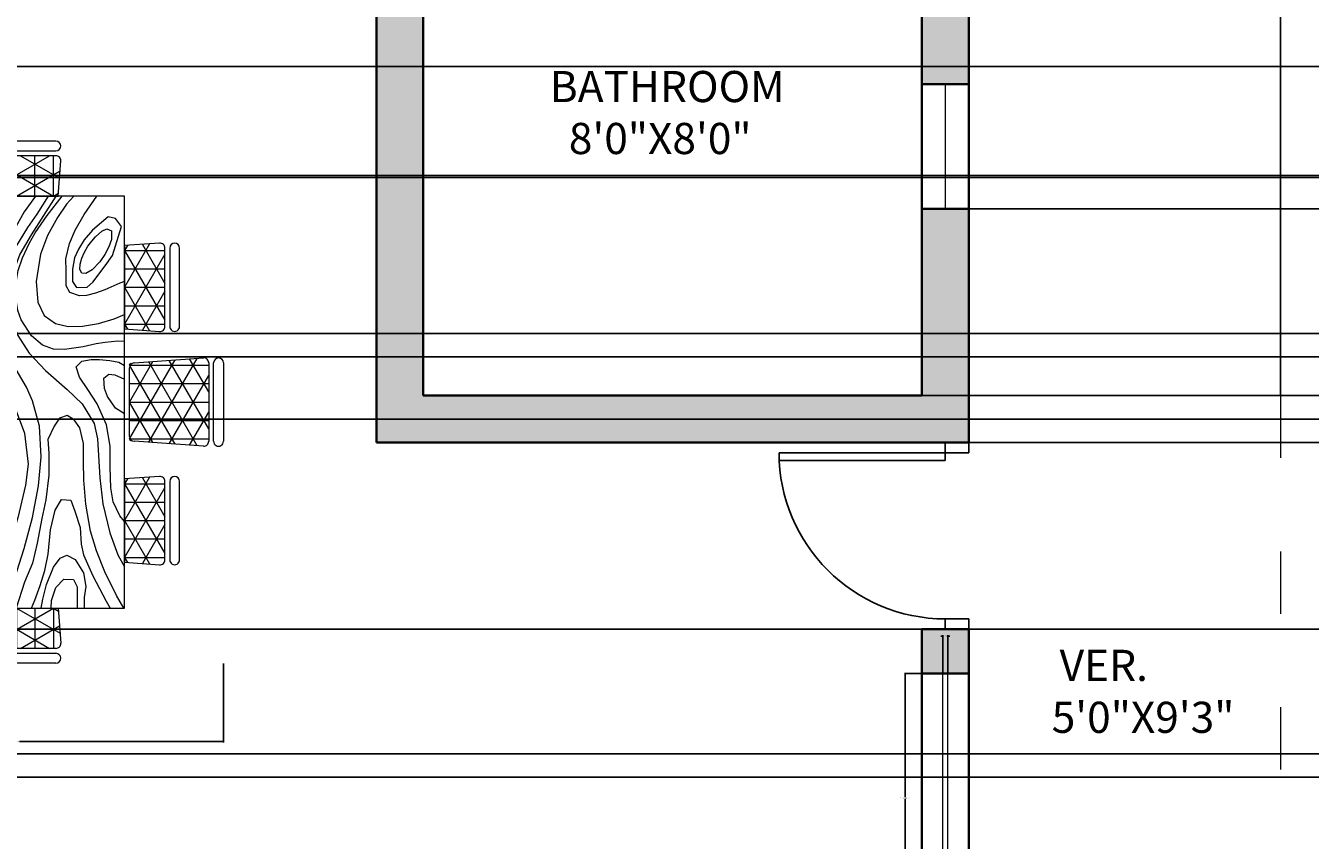
# Model space of a CAD drawing. Units: inches. Extents: x 5716 to 6907, y 12769 to 13594.
# Tile 8 of 17: x 6007 to 6254, y 13109 to 13265. Entities that reach past the tile are written whole.
import ezdxf

# ---------------------------------------------------------------- set-up
doc = ezdxf.new("R2010")
doc.units = ezdxf.units.IN
doc.linetypes.add('ACAD_ISO03W100', pattern=[30, 12, -18])
for name, color, linetype, lineweight in [('A-ANNO-DIMS', 2, 'Continuous', 18), ('A-AREA-IDEN', 7, 'Continuous', 18), ('A-DOOR', 4, 'Continuous', 25), ('A-FLOR-OVHD', 8, 'ACAD_ISO03W100', 18), ('A-FURN', 8, 'Continuous', 18), ('A-GLAZ', 4, 'Continuous', 18), ('A-WALL', 7, 'Continuous', 35), ('A-WALL-PATT', 252, 'Continuous', 13)]:
    doc.layers.add(name, color=color, linetype=linetype, lineweight=lineweight)
doc.styles.get("Standard").update_dxf_attribs({"font": 'arial.ttf'})
doc.dimstyles.get("Standard").update_dxf_attribs({"dimtxt": 0.18, "dimasz": 0.18, "dimexe": 0.18, "dimexo": 0.0625, "dimgap": 0.09, "dimtad": 0, "dimtih": 1, "dimtoh": 1, "dimdec": 4, "dimzin": 0, "dimdsep": 46, "dimtxsty": 'Standard', "dimcen": 0.09, "dimadec": 0, "dimazin": 0, "dimtfac": 1, "dimtdec": 4, "dimtofl": 0, "dimtmove": 0, "dimatfit": 3, "dimfxl": 1, "dimtolj": 1, "dimtzin": 0, "dimarcsym": 0})

# ---------------------------------------------------------------- blocks, each defined once
blk = doc.blocks.new('A$C405465A0')
for p, q in [((1.1305, 2.1034), (1.5301, 2.1034)), ((1.279, 2.0284), (1.1105, 1.9312)), ((1.4665, 2.0284), (1.1178, 1.8271)), ((1.5301, 2.0534), (1.1305, 2.0534)), ((1.1305, 2.0284), (1.5301, 2.0284)), ((1.1428, 1.625), (1.1428, 2.0284)), ((1.5427, 1.8271), (1.1941, 2.0284)), ((1.2365, 1.625), (1.2365, 2.0284)), ((1.3303, 1.625), (1.3303, 2.0284)), ((1.5501, 1.9312), (1.3816, 2.0284)), ((1.424, 1.625), (1.424, 2.0284)), ((1.5178, 1.625), (1.5178, 2.0284)), ((1.1304, 1.6481), (1.1055, 2.0017)), ((1.5354, 1.7231), (1.1078, 1.97)), ((1.5528, 1.97), (1.1252, 1.7231)), ((1.555, 2.0017), (1.5301, 1.6481)), ((0.9452, 1.8803), (0.5455, 1.8803)), ((1.5178, 1.625), (1.1157, 1.8572)), ((1.5449, 1.8572), (1.1428, 1.625)), ((2.1342, 1.8803), (1.7345, 1.8803)), ((0.5206, 1.7786), (0.5332, 1.6)), ((0.5268, 1.6904), (0.7259, 1.8053)), ((0.5455, 1.8303), (0.9452, 1.8303)), ((0.9452, 1.8053), (0.5455, 1.8053)), ((0.5578, 1.6), (0.5578, 1.8053)), ((0.5578, 1.6), (0.9134, 1.8053)), ((0.5773, 1.8053), (0.9328, 1.6)), ((0.6516, 1.6), (0.6516, 1.8053)), ((0.7453, 1.6), (0.7453, 1.8053)), ((0.7648, 1.8053), (0.9639, 1.6904)), ((0.8391, 1.6), (0.8391, 1.8053)), ((0.9328, 1.6), (0.9328, 1.8053)), ((0.9575, 1.6), (0.9701, 1.7786)), ((1.7096, 1.7786), (1.7222, 1.6)), ((1.7158, 1.6904), (1.9149, 1.8053)), ((1.7345, 1.8303), (2.1342, 1.8303)), ((2.1342, 1.8053), (1.7345, 1.8053)), ((1.7468, 1.6), (1.7468, 1.8053)), ((1.7468, 1.6), (2.1024, 1.8053)), ((1.7663, 1.8053), (2.1218, 1.6)), ((1.8406, 1.6), (1.8406, 1.8053)), ((1.9343, 1.6), (1.9343, 1.8053)), ((1.9538, 1.8053), (2.1529, 1.6904)), ((2.0281, 1.6), (2.0281, 1.8053)), ((2.1218, 1.6), (2.1218, 1.8053)), ((2.1465, 1.6), (2.1591, 1.7786)), ((0.5242, 1.7277), (0.7453, 1.6)), ((0.7453, 1.6), (0.9665, 1.7277)), ((1.3303, 1.625), (1.1237, 1.7443)), ((1.5369, 1.7443), (1.3303, 1.625)), ((1.7132, 1.7277), (1.9343, 1.6)), ((1.9343, 1.6), (2.1555, 1.7277)), ((2.3803, 1.6), (0.2803, 1.6)), ((0.2803, 1.6), (0.2803, 0.5)), ((0.4356, 1.5842), (0.3956, 1.553)), ((0.5827, 1.5379), (0.4356, 1.5842)), ((0.5321, 1.6149), (0.5578, 1.6)), ((0.5332, 1.6), (0.9575, 1.6)), ((0.7152, 1.6), (0.7236, 1.5766)), ((0.7236, 1.5766), (0.7578, 1.4998)), ((0.9055, 1.5469), (0.8836, 1.6)), ((0.9328, 1.6), (0.9586, 1.6149)), ((1.0212, 1.6), (1.0194, 1.5656)), ((1.1178, 1.5243), (1.1269, 1.5706)), ((1.1269, 1.5706), (1.1432, 1.6)), ((1.1428, 1.625), (1.1316, 1.6315)), ((1.5052, 1.625), (1.1554, 1.625)), ((1.1922, 1.5507), (1.214, 1.6)), ((1.3907, 1.6), (1.3616, 1.5541)), ((1.529, 1.6315), (1.5178, 1.625)), ((1.7211, 1.6149), (1.7468, 1.6)), ((1.7222, 1.6), (2.1465, 1.6)), ((1.9093, 1.5754), (1.8386, 1.5427)), ((1.9386, 1.6), (1.9093, 1.5754)), ((2.1086, 1.5664), (2.17, 1.6)), ((2.1218, 1.6), (2.1476, 1.6149)), ((2.3803, 1.5967), (2.3153, 1.558)), ((2.3803, 0.5), (2.3803, 1.6)), ((0.3956, 1.553), (0.3856, 1.5163)), ((0.3856, 1.5163), (0.4538, 1.4363)), ((0.4482, 1.5094), (0.4582, 1.5336)), ((0.4595, 1.4847), (0.4482, 1.5094)), ((0.4582, 1.5336), (0.5016, 1.5339)), ((0.5016, 1.5339), (0.54, 1.5204)), ((0.54, 1.5204), (0.5786, 1.5)), ((0.6365, 1.5019), (0.5827, 1.5379)), ((0.9296, 1.4669), (0.9055, 1.5469)), ((1.0194, 1.5656), (1.026, 1.5003)), ((1.1128, 1.4699), (1.1178, 1.5243)), ((1.1887, 1.5196), (1.1922, 1.5507)), ((1.2089, 1.4946), (1.1887, 1.5196)), ((1.3027, 1.5125), (1.2618, 1.4976)), ((1.3616, 1.5541), (1.3027, 1.5125)), ((1.446, 1.5079), (1.3392, 1.4609)), ((1.5543, 1.5261), (1.446, 1.5079)), ((1.6627, 1.5271), (1.5543, 1.5261)), ((1.7679, 1.5301), (1.6627, 1.5271)), ((1.8386, 1.5427), (1.7679, 1.5301)), ((1.8488, 1.4892), (1.9962, 1.5248)), ((1.9962, 1.5248), (2.1086, 1.5664)), ((2.3153, 1.558), (2.1962, 1.4994)), ((2.215, 1.4381), (2.3447, 1.5068)), ((2.3447, 1.5068), (2.3803, 1.5269)), ((0.3744, 1.3943), (0.2803, 1.458)), ((0.4876, 1.4521), (0.4595, 1.4847)), ((0.5099, 1.4328), (0.4876, 1.4521)), ((0.5786, 1.5), (0.6151, 1.4744)), ((0.6151, 1.4744), (0.6557, 1.4351)), ((0.7193, 1.4377), (0.6365, 1.5019)), ((0.7578, 1.4998), (0.7752, 1.4525)), ((0.7752, 1.4525), (0.7871, 1.4053)), ((0.9436, 1.385), (0.9296, 1.4669)), ((1.026, 1.5003), (1.0343, 1.4559)), ((1.0343, 1.4559), (1.0488, 1.3883)), ((1.1133, 1.4295), (1.1128, 1.4699)), ((1.2618, 1.4976), (1.2089, 1.4946)), ((1.3392, 1.4609), (1.2655, 1.4131)), ((1.3398, 1.3841), (1.4396, 1.445)), ((1.4396, 1.445), (1.5179, 1.4625)), ((1.5179, 1.4625), (1.717, 1.474)), ((1.717, 1.474), (1.8488, 1.4892)), ((2.0887, 1.4564), (1.9879, 1.4268)), ((2.1962, 1.4994), (2.0887, 1.4564)), ((0.4543, 1.3479), (0.3744, 1.3943)), ((0.4538, 1.4363), (0.5034, 1.394)), ((0.5034, 1.394), (0.551, 1.3648)), ((0.5366, 1.4137), (0.5099, 1.4328)), ((0.5694, 1.3947), (0.5366, 1.4137)), ((0.597, 1.3823), (0.5694, 1.3947)), ((0.6281, 1.3731), (0.597, 1.3823)), ((0.674, 1.3825), (0.654, 1.3714)), ((0.6557, 1.4351), (0.6746, 1.4025)), ((0.6746, 1.4025), (0.674, 1.3825)), ((0.7442, 1.4091), (0.7193, 1.4377)), ((0.746, 1.3555), (0.7442, 1.4091)), ((0.7871, 1.4053), (0.7898, 1.3706)), ((0.9447, 1.3133), (0.9436, 1.385)), ((1.0488, 1.3883), (1.0626, 1.2943)), ((1.1222, 1.3821), (1.1133, 1.4295)), ((1.1508, 1.3537), (1.1222, 1.3821)), ((1.2655, 1.4131), (1.2034, 1.3712)), ((1.2659, 1.3078), (1.3398, 1.3841)), ((1.5407, 1.3902), (1.4616, 1.3726)), ((1.6315, 1.3907), (1.5407, 1.3902)), ((1.7291, 1.3922), (1.6315, 1.3907)), ((1.8502, 1.4019), (1.7291, 1.3922)), ((1.9879, 1.4268), (1.8502, 1.4019)), ((1.9689, 1.3731), (2.0551, 1.3789)), ((2.0551, 1.3789), (2.1089, 1.3912)), ((2.1089, 1.3912), (2.215, 1.4381)), ((2.1327, 1.3477), (2.1998, 1.3905)), ((2.1998, 1.3905), (2.271, 1.4021)), ((2.271, 1.4021), (2.3264, 1.3943)), ((2.3264, 1.3943), (2.3803, 1.3943)), ((0.2803, 1.3424), (0.3226, 1.3046)), ((0.523, 1.3203), (0.4543, 1.3479)), ((0.6007, 1.301), (0.523, 1.3203)), ((0.551, 1.3648), (0.5952, 1.3458)), ((0.5952, 1.3458), (0.6524, 1.335)), ((0.654, 1.3714), (0.6281, 1.3731)), ((0.6524, 1.335), (0.7159, 1.3352)), ((0.7159, 1.3352), (0.746, 1.3555)), ((0.7722, 1.3216), (0.7385, 1.3018)), ((0.7898, 1.3706), (0.7722, 1.3216)), ((0.9305, 1.2479), (0.9447, 1.3133)), ((1.2034, 1.3712), (1.1508, 1.3537)), ((1.4211, 1.3426), (1.398, 1.3071)), ((1.4616, 1.3726), (1.4211, 1.3426)), ((1.8267, 1.2783), (1.8309, 1.3257)), ((1.8309, 1.3257), (1.8869, 1.3472)), ((1.8869, 1.3472), (1.9689, 1.3731)), ((2.1112, 1.3052), (2.1327, 1.3477)), ((2.2336, 1.2914), (2.2346, 1.3391)), ((2.2346, 1.3391), (2.2726, 1.3593)), ((2.2726, 1.3593), (2.339, 1.3581)), ((2.339, 1.3581), (2.3803, 1.3581)), ((0, 1.2499), (0, 0.8502)), ((0.05, 0.8502), (0.05, 1.2499)), ((0.075, 1.0695), (0.19, 1.2686)), ((0.075, 1.2499), (0.075, 0.8502)), ((0.2803, 1.2622), (0.1018, 1.2748)), ((0.2803, 1.05), (0.1526, 1.2712)), ((0.2803, 1.2375), (0.2654, 1.2633)), ((0.3797, 1.2052), (0.2803, 1.2816)), ((0.2803, 0.8379), (0.2803, 1.2622)), ((0.2803, 1.2498), (0.478, 1.1251)), ((0.3226, 1.3046), (0.3891, 1.2586)), ((0.3891, 1.2586), (0.4808, 1.2074)), ((0.6623, 1.3018), (0.6007, 1.301)), ((0.7385, 1.3018), (0.6623, 1.3018)), ((0.8894, 1.1911), (0.9305, 1.2479)), ((1.0626, 1.2943), (1.06, 1.2384)), ((1.1689, 1.1968), (1.2659, 1.3078)), ((1.398, 1.3071), (1.412, 1.2681)), ((1.412, 1.2681), (1.4535, 1.2416)), ((1.8814, 1.2462), (1.8267, 1.2783)), ((1.9819, 1.2225), (1.8814, 1.2462)), ((2.1264, 1.2714), (2.1112, 1.3052)), ((2.171, 1.2386), (2.1264, 1.2714)), ((2.2746, 1.2504), (2.2336, 1.2914)), ((2.3417, 1.2285), (2.2746, 1.2504)), ((2.3803, 1.2622), (2.5588, 1.2748)), ((2.3803, 1.05), (2.508, 1.2712)), ((2.3803, 1.2375), (2.3951, 1.2633)), ((2.3803, 0.8379), (2.3803, 1.2622)), ((2.5856, 1.0695), (2.4706, 1.2686)), ((2.5856, 1.2499), (2.5856, 0.8502)), ((2.6106, 0.8502), (2.6106, 1.2499)), ((2.6606, 1.2499), (2.6606, 0.8502)), ((0.2803, 1.2375), (0.075, 1.2375)), ((0.075, 0.882), (0.2803, 1.2375)), ((0.2803, 0.8625), (0.075, 1.2181)), ((0.3728, 1.1548), (0.2803, 1.2123)), ((0.4682, 1.1454), (0.3797, 1.2052)), ((0.4808, 1.2074), (0.5771, 1.1712)), ((0.8213, 1.159), (0.8894, 1.1911)), ((1.0402, 1.1815), (0.9932, 1.1252)), ((1.06, 1.2384), (1.0402, 1.1815)), ((1.0809, 1.1136), (1.1689, 1.1968)), ((1.4535, 1.2416), (1.5203, 1.2085)), ((1.5203, 1.2085), (1.5912, 1.2143)), ((1.5912, 1.2143), (1.7027, 1.2151)), ((1.7027, 1.2151), (1.8282, 1.1987)), ((1.8282, 1.1987), (1.9236, 1.1792)), ((1.9236, 1.1792), (2.049, 1.1552)), ((2.1048, 1.2108), (1.9819, 1.2225)), ((2.1888, 1.194), (2.1048, 1.2108)), ((2.2593, 1.2028), (2.171, 1.2386)), ((2.2653, 1.1704), (2.1888, 1.194)), ((2.3339, 1.1841), (2.2593, 1.2028)), ((2.3803, 1.1754), (2.3339, 1.1841)), ((2.3803, 1.226), (2.3417, 1.2285)), ((2.3803, 1.2375), (2.5856, 1.2375)), ((2.5856, 0.882), (2.3803, 1.2375)), ((2.3803, 0.8625), (2.5856, 1.2181)), ((0.2803, 1.1438), (0.075, 1.1438)), ((0.2803, 1.1471), (0.3609, 1.0879)), ((0.4405, 1.1078), (0.3728, 1.1548)), ((0.5225, 1.114), (0.4682, 1.1454)), ((0.478, 1.1251), (0.576, 1.067)), ((0.5954, 1.0801), (0.5225, 1.114)), ((0.5771, 1.1712), (0.7161, 1.1491)), ((0.7161, 1.1491), (0.8213, 1.159)), ((0.9932, 1.1252), (0.9121, 1.0739)), ((0.9908, 1.0561), (1.0809, 1.1136)), ((1.3237, 1.1316), (1.2549, 1.1012)), ((1.4537, 1.1662), (1.3237, 1.1316)), ((1.6097, 1.1755), (1.4537, 1.1662)), ((1.757, 1.1624), (1.6097, 1.1755)), ((1.9184, 1.131), (1.757, 1.1624)), ((2.0769, 1.0887), (1.9184, 1.131)), ((2.049, 1.1552), (2.1515, 1.1303)), ((2.1515, 1.1303), (2.2486, 1.0908)), ((2.3396, 1.1432), (2.2653, 1.1704)), ((2.3803, 1.126), (2.3396, 1.1432)), ((2.3803, 1.1438), (2.5856, 1.1438)), ((0.2803, 1.05), (0.075, 1.05)), ((0.1526, 0.8289), (0.2803, 1.05)), ((0.3609, 1.0879), (0.5015, 1.0099)), ((0.5402, 1.0464), (0.4405, 1.1078)), ((0.576, 1.067), (0.7146, 1.0163)), ((0.6603, 1.0585), (0.5954, 1.0801)), ((0.7308, 1.0454), (0.6603, 1.0585)), ((0.863, 1.056), (0.7897, 1.0439)), ((0.9121, 1.0739), (0.863, 1.056)), ((0.9069, 1.0237), (0.9908, 1.0561)), ((1.2549, 1.1012), (1.1432, 1.0368)), ((1.2543, 0.9907), (1.3755, 1.0479)), ((1.3755, 1.0479), (1.4887, 1.0901)), ((1.4887, 1.0901), (1.6473, 1.1088)), ((1.6473, 1.1088), (1.7544, 1.0961)), ((1.7544, 1.0961), (1.9207, 1.0564)), ((1.9207, 1.0564), (2.1244, 0.9922)), ((2.2686, 1.0282), (2.0769, 1.0887)), ((2.2486, 1.0908), (2.3803, 1.048)), ((2.3803, 1.05), (2.5856, 1.05)), ((2.508, 0.8289), (2.3803, 1.05)), ((0.19, 0.8315), (0.075, 1.0306)), ((0.3078, 1.029), (0.2803, 1.0458)), ((0.346, 1.0052), (0.3078, 1.029)), ((0.4051, 0.9771), (0.346, 1.0052)), ((0.5015, 1.0099), (0.6086, 0.961)), ((0.6261, 1.0028), (0.5402, 1.0464)), ((0.7415, 0.9604), (0.6261, 1.0028)), ((0.7146, 1.0163), (0.7979, 1.0084)), ((0.7897, 1.0439), (0.7308, 1.0454)), ((0.7979, 1.0084), (0.9069, 1.0237)), ((1.0559, 0.9876), (0.958, 0.9508)), ((1.1432, 1.0368), (1.0559, 0.9876)), ((1.1244, 0.9348), (1.2543, 0.9907)), ((2.1244, 0.9922), (2.2495, 0.9522)), ((2.3803, 0.9983), (2.2686, 1.0282)), ((2.4706, 0.8315), (2.5856, 1.0306)), ((0.2803, 0.9563), (0.075, 0.9563)), ((0.309, 0.9074), (0.2803, 0.9224)), ((0.4579, 0.9575), (0.4051, 0.9771)), ((0.5195, 0.9378), (0.4579, 0.9575)), ((0.5818, 0.918), (0.5195, 0.9378)), ((0.6352, 0.8954), (0.5818, 0.918)), ((0.6086, 0.961), (0.7339, 0.9201)), ((0.7339, 0.9201), (0.8463, 0.9008)), ((0.8579, 0.9417), (0.7415, 0.9604)), ((0.958, 0.9508), (0.8579, 0.9417)), ((0.9714, 0.9002), (1.1244, 0.9348)), ((1.301, 0.9003), (1.4378, 0.9282)), ((1.4378, 0.9282), (1.5224, 0.9439)), ((1.5224, 0.9439), (1.6187, 0.9581)), ((1.6187, 0.9581), (1.7607, 0.9676)), ((1.7607, 0.9676), (1.9339, 0.9563)), ((1.9339, 0.9563), (2.0478, 0.9301)), ((2.0478, 0.9301), (2.1209, 0.9013)), ((2.2495, 0.9522), (2.3803, 0.9025)), ((2.3803, 0.9563), (2.5856, 0.9563)), ((0.2803, 0.8625), (0.075, 0.8625)), ((0.2654, 0.8368), (0.2803, 0.8625)), ((0.342, 0.8943), (0.309, 0.9074)), ((0.3823, 0.8837), (0.342, 0.8943)), ((0.4349, 0.876), (0.3823, 0.8837)), ((0.4843, 0.8652), (0.4349, 0.876)), ((0.5229, 0.85), (0.4843, 0.8652)), ((0.6712, 0.8671), (0.6352, 0.8954)), ((0.6805, 0.8424), (0.6712, 0.8671)), ((0.8463, 0.9008), (0.9714, 0.9002)), ((0.9468, 0.8025), (1.1125, 0.8545)), ((1.1125, 0.8545), (1.224, 0.8829)), ((1.224, 0.8829), (1.301, 0.9003)), ((1.5313, 0.864), (1.3995, 0.834)), ((1.6341, 0.8806), (1.5313, 0.864)), ((1.7415, 0.8904), (1.6341, 0.8806)), ((1.8296, 0.8853), (1.7415, 0.8904)), ((1.9317, 0.8609), (1.8296, 0.8853)), ((2.0406, 0.8138), (1.9317, 0.8609)), ((2.1209, 0.9013), (2.214, 0.8459)), ((2.3803, 0.8625), (2.5856, 0.8625)), ((2.3951, 0.8368), (2.3803, 0.8625)), ((0.1018, 0.8253), (0.2803, 0.8379)), ((0.5441, 0.8372), (0.5229, 0.85)), ((0.5622, 0.8164), (0.5441, 0.8372)), ((0.5562, 0.7809), (0.5634, 0.7968)), ((0.5634, 0.7968), (0.5622, 0.8164)), ((0.6434, 0.7666), (0.675, 0.8159)), ((0.675, 0.8159), (0.6805, 0.8424)), ((0.8288, 0.7556), (0.9468, 0.8025)), ((1.2818, 0.7979), (1.131, 0.7357)), ((1.3995, 0.834), (1.2818, 0.7979)), ((1.4547, 0.7504), (1.6229, 0.7863)), ((1.6229, 0.7863), (1.7436, 0.7907)), ((1.7436, 0.7907), (1.8858, 0.7711)), ((2.1229, 0.7618), (2.0406, 0.8138)), ((2.214, 0.8459), (2.297, 0.7736)), ((2.5588, 0.8253), (2.3803, 0.8379)), ((0.4801, 0.7185), (0.5313, 0.7537)), ((0.5313, 0.7537), (0.5562, 0.7809)), ((0.5568, 0.6828), (0.603, 0.7231)), ((0.603, 0.7231), (0.6434, 0.7666)), ((0.6995, 0.6921), (0.8288, 0.7556)), ((1.131, 0.7357), (0.9946, 0.6604)), ((1.2995, 0.6899), (1.4547, 0.7504)), ((1.8858, 0.7711), (1.9957, 0.7333)), ((1.9957, 0.7333), (2.0772, 0.6873)), ((2.1698, 0.724), (2.1229, 0.7618)), ((2.2541, 0.6328), (2.1698, 0.724)), ((2.297, 0.7736), (2.3432, 0.7176)), ((0.2803, 0.6573), (0.312, 0.6622)), ((0.312, 0.6622), (0.3723, 0.6742)), ((0.3723, 0.6742), (0.4317, 0.6944)), ((0.4317, 0.6944), (0.4801, 0.7185)), ((0.499, 0.6426), (0.5568, 0.6828)), ((0.6181, 0.6464), (0.6995, 0.6921)), ((0.9946, 0.6604), (0.8746, 0.5766)), ((1.2062, 0.6433), (1.2995, 0.6899)), ((1.4124, 0.6631), (1.3518, 0.6302)), ((1.4772, 0.6838), (1.4124, 0.6631)), ((1.554, 0.696), (1.4772, 0.6838)), ((1.5115, 0.6388), (1.5744, 0.6543)), ((1.6333, 0.6993), (1.554, 0.696)), ((1.5744, 0.6543), (1.6677, 0.668)), ((1.7153, 0.696), (1.6333, 0.6993)), ((1.6677, 0.668), (1.7434, 0.6684)), ((1.7865, 0.6892), (1.7153, 0.696)), ((1.7434, 0.6684), (1.8417, 0.6617)), ((1.8794, 0.6748), (1.7865, 0.6892)), ((1.8417, 0.6617), (1.8785, 0.6547)), ((1.8785, 0.6547), (1.9243, 0.6434)), ((1.9674, 0.6548), (1.8794, 0.6748)), ((2.0494, 0.621), (1.9674, 0.6548)), ((2.0772, 0.6873), (2.1261, 0.6491)), ((2.3432, 0.7176), (2.3803, 0.6555)), ((0.3813, 0.5837), (0.4497, 0.615)), ((0.4385, 0.5349), (0.5546, 0.6082)), ((0.4497, 0.615), (0.499, 0.6426)), ((0.5546, 0.6082), (0.6181, 0.6464)), ((1.1078, 0.5882), (1.2062, 0.6433)), ((1.3133, 0.5983), (1.2908, 0.5736)), ((1.3518, 0.6302), (1.3133, 0.5983)), ((1.3959, 0.5264), (1.4712, 0.6079)), ((1.4712, 0.6079), (1.5115, 0.6388)), ((1.4736, 0.5658), (1.4828, 0.5927)), ((1.4828, 0.5927), (1.5188, 0.6159)), ((1.5188, 0.6159), (1.6031, 0.6361)), ((1.5621, 0.583), (1.5815, 0.6002)), ((1.5815, 0.6002), (1.641, 0.6183)), ((1.6031, 0.6361), (1.6918, 0.6436)), ((1.641, 0.6183), (1.6861, 0.6235)), ((1.6861, 0.6235), (1.7353, 0.624)), ((1.6918, 0.6436), (1.8075, 0.6404)), ((1.7353, 0.624), (1.7765, 0.6204)), ((1.7765, 0.6204), (1.811, 0.6136)), ((1.8075, 0.6404), (1.8682, 0.6312)), ((1.811, 0.6136), (1.8414, 0.6025)), ((1.8414, 0.6025), (1.8603, 0.5873)), ((1.8682, 0.6312), (1.909, 0.622)), ((1.909, 0.622), (1.9497, 0.5991)), ((1.9243, 0.6434), (1.9761, 0.6102)), ((1.9497, 0.5991), (1.9595, 0.5705)), ((1.9761, 0.6102), (2.006, 0.5625)), ((2.1071, 0.5697), (2.0494, 0.621)), ((2.1261, 0.6491), (2.1688, 0.6067)), ((2.1688, 0.6067), (2.197, 0.5721)), ((2.3022, 0.5551), (2.2541, 0.6328)), ((0.2803, 0.5477), (0.3159, 0.5583)), ((0.3159, 0.5583), (0.3813, 0.5837)), ((0.3857, 0.5), (0.4385, 0.5349)), ((0.8225, 0.5348), (0.7878, 0.5)), ((0.8746, 0.5766), (0.8225, 0.5348)), ((0.9657, 0.5), (1.0064, 0.5273)), ((1.0064, 0.5273), (1.1078, 0.5882)), ((1.2908, 0.5736), (1.2556, 0.52)), ((1.3784, 0.5), (1.3959, 0.5264)), ((1.4775, 0.5489), (1.4736, 0.5658)), ((1.5273, 0.534), (1.4775, 0.5489)), ((1.6327, 0.513), (1.5273, 0.534)), ((1.572, 0.557), (1.5621, 0.583)), ((1.5997, 0.5436), (1.572, 0.557)), ((1.6329, 0.5353), (1.5997, 0.5436)), ((1.6895, 0.5294), (1.6329, 0.5353)), ((1.7388, 0.53), (1.6895, 0.5294)), ((1.7888, 0.5363), (1.7388, 0.53)), ((1.8321, 0.5488), (1.7888, 0.5363)), ((1.8611, 0.5702), (1.8321, 0.5488)), ((1.9108, 0.5271), (1.8503, 0.5169)), ((1.8603, 0.5873), (1.8611, 0.5702)), ((1.9448, 0.5456), (1.9108, 0.5271)), ((1.9595, 0.5705), (1.9448, 0.5456)), ((2.006, 0.5625), (2.0103, 0.5395)), ((2.0103, 0.5395), (2.0069, 0.5)), ((2.1338, 0.529), (2.1071, 0.5697)), ((2.1506, 0.5), (2.1338, 0.529)), ((2.197, 0.5721), (2.2242, 0.5314)), ((2.2242, 0.5314), (2.2363, 0.5)), ((2.3248, 0.5), (2.3022, 0.5551)), ((0.2803, 0.5), (2.3803, 0.5)), ((0.5126, 0.2463), (0.9147, 0.4784)), ((0.5205, 0.3591), (0.7272, 0.4784)), ((0.5285, 0.4719), (0.5397, 0.4784)), ((0.5397, 0.4784), (0.5397, 0.075)), ((0.5397, 0.4784), (0.9417, 0.2463)), ((0.5522, 0.4784), (0.9021, 0.4784)), ((0.6334, 0.4784), (0.6334, 0.075)), ((0.7272, 0.4784), (0.7272, 0.075)), ((0.7272, 0.4784), (0.9338, 0.3591)), ((0.8209, 0.4784), (0.8209, 0.075)), ((0.9147, 0.4784), (0.9147, 0.075)), ((0.9147, 0.4784), (0.9258, 0.4719)), ((1.1055, 0.3215), (1.1181, 0.5)), ((1.1091, 0.3724), (1.3303, 0.5)), ((1.1171, 0.4852), (1.1428, 0.5)), ((1.1181, 0.5), (1.5425, 0.5)), ((1.1428, 0.5), (1.1428, 0.2948)), ((1.1428, 0.5), (1.4984, 0.2948)), ((1.1622, 0.2948), (1.5178, 0.5)), ((1.2365, 0.5), (1.2365, 0.2948)), ((1.2556, 0.52), (1.2455, 0.5)), ((1.3303, 0.5), (1.3303, 0.2948)), ((1.3303, 0.5), (1.5515, 0.3724)), ((1.424, 0.5), (1.424, 0.2948)), ((1.5178, 0.5), (1.5178, 0.2948)), ((1.5178, 0.5), (1.5435, 0.4852)), ((1.5425, 0.5), (1.555, 0.3215)), ((1.685, 0.5094), (1.6327, 0.513)), ((1.7331, 0.5091), (1.685, 0.5094)), ((1.7096, 0.3215), (1.7222, 0.5)), ((1.7132, 0.3724), (1.9343, 0.5)), ((1.7211, 0.4852), (1.7468, 0.5)), ((1.7222, 0.5), (2.1465, 0.5)), ((1.7906, 0.5103), (1.7331, 0.5091)), ((1.7468, 0.5), (1.7468, 0.2948)), ((1.7468, 0.5), (2.1024, 0.2948)), ((1.7663, 0.2948), (2.1218, 0.5)), ((1.8503, 0.5169), (1.7906, 0.5103)), ((1.8406, 0.5), (1.8406, 0.2948)), ((1.9343, 0.5), (1.9343, 0.2948)), ((1.9343, 0.5), (2.1555, 0.3724)), ((2.0281, 0.5), (2.0281, 0.2948)), ((2.1218, 0.5), (2.1218, 0.2948)), ((2.1218, 0.5), (2.1476, 0.4852)), ((2.1465, 0.5), (2.1591, 0.3215)), ((0.5024, 0.1018), (0.5273, 0.4553)), ((0.927, 0.4553), (0.9519, 0.1018)), ((1.1118, 0.4097), (1.3109, 0.2948)), ((1.3497, 0.2948), (1.5488, 0.4097)), ((1.7158, 0.4097), (1.9149, 0.2948)), ((1.9538, 0.2948), (2.1529, 0.4097)), ((0.5046, 0.1334), (0.9323, 0.3803)), ((0.522, 0.3803), (0.9497, 0.1334)), ((0.5147, 0.2763), (0.8634, 0.075)), ((0.591, 0.075), (0.9396, 0.2763)), ((1.5301, 0.2948), (1.1305, 0.2948)), ((1.1305, 0.2698), (1.5301, 0.2698)), ((2.1342, 0.2948), (1.7345, 0.2948)), ((1.7345, 0.2698), (2.1342, 0.2698)), ((1.5301, 0.2198), (1.1305, 0.2198)), ((2.1342, 0.2198), (1.7345, 0.2198)), ((0.5074, 0.1723), (0.6759, 0.075)), ((0.7785, 0.075), (0.9469, 0.1723)), ((0.927, 0.075), (0.5273, 0.075)), ((0.5273, 0.05), (0.927, 0.05)), ((0.927, 0), (0.5273, 0))]:
    blk.add_line(p, q)
for centre, start, end in [((1.1305, 2.0784), 90, 270), ((1.5301, 2.0784), 270, 90), ((1.1305, 2.0034), 90, 184.02744), ((1.5301, 2.0034), 355.97256, 90), ((0.5455, 1.8553), 90, 270), ((0.9452, 1.8553), 270, 90), ((1.7345, 1.8553), 90, 270), ((2.1342, 1.8553), 270, 90), ((0.5455, 1.7803), 90, 184.02744), ((0.9452, 1.7803), 355.97256, 90), ((1.7345, 1.7803), 90, 184.02744), ((2.1342, 1.7803), 355.97256, 90), ((1.1554, 1.65), 184.39871, 270), ((1.5052, 1.65), 270, 355.60129), ((0.025, 1.2499), 0, 180), ((0.1, 1.2499), 85.97256, 180), ((2.5606, 1.2499), 0, 94.02744), ((2.6356, 1.2499), 0, 180), ((0.025, 0.8502), 180, 0), ((0.1, 0.8502), 180, 274.02744), ((2.5606, 0.8502), 265.97256, 0), ((2.6356, 0.8502), 180, 0), ((0.5522, 0.4534), 90, 175.60129), ((0.9021, 0.4534), 4.39871, 90), ((1.1305, 0.3198), 175.97256, 270), ((1.1305, 0.2448), 90, 270), ((1.5301, 0.3198), 270, 4.02744), ((1.5301, 0.2448), 270, 90), ((1.7345, 0.3198), 175.97256, 270), ((1.7345, 0.2448), 90, 270), ((2.1342, 0.3198), 270, 4.02744), ((2.1342, 0.2448), 270, 90), ((0.5273, 0.1), 175.97256, 270), ((0.927, 0.1), 270, 4.02744), ((0.5273, 0.025), 90, 270), ((0.927, 0.025), 270, 90)]:
    blk.add_arc(centre, 0.025, start, end)
blk = doc.blocks.new('DOOR-SWING-36IN')
for p, q in [((0, 32), (0, 0)), ((1.5, 31.96), (1.5, 0)), ((-2, 0), (0, 0)), ((0, 0), (0, -4.5)), ((0, 0), (1.5, 0)), ((34, 0), (32, 0)), ((32, 0), (32, -4.5)), ((0, -4.5), (-2, -4.5)), ((32, -4.5), (34, -4.5))]:
    blk.add_line(p, q)
blk.add_arc((0, 0), 32, 0, 90)
blk = doc.blocks.new('WIN-GLAZING-48IN')
for p, q in [((0, 0), (0, 48)), ((1, 0), (1, 48))]:
    blk.add_line(p, q)
blk = doc.blocks.new('*D31')
at = {"layer": 'A-ANNO-DIMS', "color": 0, "lineweight": -2, "transparency": 16777216}
for p, q in [((6182.96, 13140.65), (6175.64, 13140.65)), ((6175.82, 13140.47), (6175.82, 13116.83)), ((6175.82, 13092.83), (6175.82, 13116.47)), ((6182.96, 13092.65), (6175.64, 13092.65))]:
    blk.add_line(p, q, dxfattribs=at)
at = {"layer": 'A-ANNO-DIMS', "color": 0, "transparency": 16777216}
for points in [[(6175.79, 13140.47), (6175.85, 13140.47), (6175.82, 13140.65)], [(6175.79, 13092.83), (6175.85, 13092.83), (6175.82, 13092.65)]]:
    blk.add_solid(points, dxfattribs=at)
at = {"layer": 'Defpoints', "color": 0, "transparency": 16777216}
for p in [(6175.82, 13140.65), (6183.02, 13140.65), (6183.02, 13092.65)]:
    blk.add_point(p, dxfattribs=at)
at = {"layer": 'A-ANNO-DIMS', "color": 0, "transparency": 16777216, "insert": (6175.82, 13116.65), "char_height": 0.18, "attachment_point": 5}
blk.add_mtext('\\A1;WINDOW 48 TYP.', dxfattribs=at)
blk = doc.blocks.new('*D32')
at = {"layer": 'A-ANNO-DIMS', "color": 0, "lineweight": -2, "transparency": 16777216}
for p, q in [((6182.84, 13147.85), (6182.66, 13147.85)), ((6183.02, 13140.71), (6183.02, 13148.03)), ((6184.02, 13140.71), (6184.02, 13148.03)), ((6184.2, 13147.85), (6184.38, 13147.85))]:
    blk.add_line(p, q, dxfattribs=at)
at = {"layer": 'A-ANNO-DIMS', "color": 0, "transparency": 16777216}
for points in [[(6182.84, 13147.88), (6182.84, 13147.82), (6183.02, 13147.85)], [(6184.2, 13147.88), (6184.2, 13147.82), (6184.02, 13147.85)]]:
    blk.add_solid(points, dxfattribs=at)
at = {"layer": 'Defpoints', "color": 0, "transparency": 16777216}
for p in [(6184.02, 13147.85), (6183.02, 13140.65), (6184.02, 13140.65)]:
    blk.add_point(p, dxfattribs=at)
at = {"layer": 'A-ANNO-DIMS', "color": 0, "transparency": 16777216, "insert": (6183.52, 13147.85), "char_height": 0.18, "attachment_point": 5}
blk.add_mtext('\\A1;1 TYP.', dxfattribs=at)
blk = doc.blocks.new('*D38')
at = {"layer": 'A-ANNO-DIMS', "color": 0, "lineweight": -2, "transparency": 16777216}
for p, q in [((5965.08, 13142.58), (5965.08, 13127.37)), ((6044.58, 13142.58), (6044.58, 13127.37)), ((5965.26, 13127.55), (6004.3, 13127.55)), ((6044.4, 13127.55), (6005.36, 13127.55))]:
    blk.add_line(p, q, dxfattribs=at)
at = {"layer": 'A-ANNO-DIMS', "color": 0, "transparency": 16777216}
for points in [[(5965.26, 13127.58), (5965.26, 13127.52), (5965.08, 13127.55)], [(6044.4, 13127.58), (6044.4, 13127.52), (6044.58, 13127.55)]]:
    blk.add_solid(points, dxfattribs=at)
at = {"layer": 'Defpoints', "color": 0, "transparency": 16777216}
for p in [(5965.08, 13142.64), (6044.58, 13142.64), (6044.58, 13127.55)]:
    blk.add_point(p, dxfattribs=at)
at = {"layer": 'A-ANNO-DIMS', "color": 0, "transparency": 16777216, "insert": (6004.83, 13127.55), "char_height": 0.18, "attachment_point": 5}
blk.add_mtext('\\A1;80 TYP.', dxfattribs=at)
blk = doc.blocks.new('*D51')
at = {"layer": 'A-ANNO-DIMS', "color": 0, "lineweight": -2, "transparency": 16777216}
for p, q in [((5819.02, 13440.21), (5819.02, 13594.38)), ((5819.2, 13594.2), (6033.23, 13594.2)), ((6247.84, 13594.2), (6033.82, 13594.2)), ((6248.02, 13194.21), (6248.02, 13594.38))]:
    blk.add_line(p, q, dxfattribs=at)
at = {"layer": 'A-ANNO-DIMS', "color": 0, "transparency": 16777216}
for points in [[(5819.2, 13594.23), (5819.2, 13594.17), (5819.02, 13594.2)], [(6247.84, 13594.23), (6247.84, 13594.17), (6248.02, 13594.2)]]:
    blk.add_solid(points, dxfattribs=at)
at = {"layer": 'Defpoints', "color": 0, "transparency": 16777216}
for p in [(6248.02, 13594.2), (5819.02, 13440.15), (6248.02, 13194.15)]:
    blk.add_point(p, dxfattribs=at)
at = {"layer": 'A-ANNO-DIMS', "color": 0, "transparency": 16777216, "insert": (6033.52, 13594.2), "char_height": 0.18, "attachment_point": 5}
blk.add_mtext('\\A1;429', dxfattribs=at)
blk = doc.blocks.new('*D52')
at = {"layer": 'A-ANNO-DIMS', "color": 0, "lineweight": -2, "transparency": 16777216}
for p, q in [((6267.34, 13440.15), (5716.04, 13440.15)), ((5716.22, 13439.97), (5716.22, 13140.83)), ((5716.22, 12841.33), (5716.22, 13140.47)), ((6267.34, 12841.15), (5716.04, 12841.15))]:
    blk.add_line(p, q, dxfattribs=at)
at = {"layer": 'A-ANNO-DIMS', "color": 0, "transparency": 16777216}
for points in [[(5716.19, 13439.97), (5716.25, 13439.97), (5716.22, 13440.15)], [(5716.19, 12841.33), (5716.25, 12841.33), (5716.22, 12841.15)]]:
    blk.add_solid(points, dxfattribs=at)
at = {"layer": 'Defpoints', "color": 0, "transparency": 16777216}
for p in [(6267.41, 13440.15), (5716.22, 12841.15), (6267.41, 12841.15)]:
    blk.add_point(p, dxfattribs=at)
at = {"layer": 'A-ANNO-DIMS', "color": 0, "transparency": 16777216, "insert": (5716.22, 13140.65), "char_height": 0.18, "attachment_point": 5}
blk.add_mtext('\\A1;599', dxfattribs=at)
blk = doc.blocks.new('*D59')
at = {"layer": 'A-ANNO-DIMS', "color": 0, "lineweight": -2, "transparency": 16777216}
for p, q in [((6736.67, 13294.65), (5716.04, 13294.65)), ((5716.22, 13294.47), (5716.22, 13248.33)), ((5716.22, 13201.83), (5716.22, 13247.97)), ((6736.67, 13201.65), (5716.04, 13201.65))]:
    blk.add_line(p, q, dxfattribs=at)
at = {"layer": 'A-ANNO-DIMS', "color": 0, "transparency": 16777216}
for points in [[(5716.19, 13294.47), (5716.25, 13294.47), (5716.22, 13294.65)], [(5716.19, 13201.83), (5716.25, 13201.83), (5716.22, 13201.65)]]:
    blk.add_solid(points, dxfattribs=at)
at = {"layer": 'Defpoints', "color": 0, "transparency": 16777216}
for p in [(6736.73, 13294.65), (5716.22, 13201.65), (6736.73, 13201.65)]:
    blk.add_point(p, dxfattribs=at)
at = {"layer": 'A-ANNO-DIMS', "color": 0, "transparency": 16777216, "insert": (5716.22, 13248.15), "char_height": 0.18, "attachment_point": 5}
blk.add_mtext('\\A1;93', dxfattribs=at)
blk = doc.blocks.new('*D60')
at = {"layer": 'A-ANNO-DIMS', "color": 0, "lineweight": -2, "transparency": 16777216}
for p, q in [((6736.67, 13201.65), (5716.04, 13201.65)), ((5716.22, 13201.47), (5716.22, 13195.83)), ((5716.22, 13189.83), (5716.22, 13195.47)), ((6827.78, 13189.65), (5716.04, 13189.65))]:
    blk.add_line(p, q, dxfattribs=at)
at = {"layer": 'A-ANNO-DIMS', "color": 0, "transparency": 16777216}
for points in [[(5716.19, 13201.47), (5716.25, 13201.47), (5716.22, 13201.65)], [(5716.19, 13189.83), (5716.25, 13189.83), (5716.22, 13189.65)]]:
    blk.add_solid(points, dxfattribs=at)
at = {"layer": 'Defpoints', "color": 0, "transparency": 16777216}
for p in [(6736.73, 13201.65), (5716.22, 13189.65), (6827.84, 13189.65)]:
    blk.add_point(p, dxfattribs=at)
at = {"layer": 'A-ANNO-DIMS', "color": 0, "transparency": 16777216, "insert": (5716.22, 13195.65), "char_height": 0.18, "attachment_point": 5}
blk.add_mtext('\\A1;12', dxfattribs=at)
blk = doc.blocks.new('*D61')
at = {"layer": 'A-ANNO-DIMS', "color": 0, "lineweight": -2, "transparency": 16777216}
for p, q in [((6827.78, 13189.65), (5716.04, 13189.65)), ((5716.22, 13189.47), (5716.22, 13155.33)), ((5716.22, 13120.83), (5716.22, 13154.97)), ((6736.67, 13120.65), (5716.04, 13120.65))]:
    blk.add_line(p, q, dxfattribs=at)
at = {"layer": 'A-ANNO-DIMS', "color": 0, "transparency": 16777216}
for points in [[(5716.19, 13189.47), (5716.25, 13189.47), (5716.22, 13189.65)], [(5716.19, 13120.83), (5716.25, 13120.83), (5716.22, 13120.65)]]:
    blk.add_solid(points, dxfattribs=at)
at = {"layer": 'Defpoints', "color": 0, "transparency": 16777216}
for p in [(6827.84, 13189.65), (5716.22, 13120.65), (6736.73, 13120.65)]:
    blk.add_point(p, dxfattribs=at)
at = {"layer": 'A-ANNO-DIMS', "color": 0, "transparency": 16777216, "insert": (5716.22, 13155.15), "char_height": 0.18, "attachment_point": 5}
blk.add_mtext('\\A1;69', dxfattribs=at)
blk = doc.blocks.new('*D62')
at = {"layer": 'A-ANNO-DIMS', "color": 0, "lineweight": -2, "transparency": 16777216}
for p, q in [((6736.67, 13120.65), (5716.04, 13120.65)), ((5716.22, 13120.47), (5716.22, 13100.33)), ((5716.22, 13079.83), (5716.22, 13099.97)), ((6736.67, 13079.65), (5716.04, 13079.65))]:
    blk.add_line(p, q, dxfattribs=at)
at = {"layer": 'A-ANNO-DIMS', "color": 0, "transparency": 16777216}
for points in [[(5716.19, 13120.47), (5716.25, 13120.47), (5716.22, 13120.65)], [(5716.19, 13079.83), (5716.25, 13079.83), (5716.22, 13079.65)]]:
    blk.add_solid(points, dxfattribs=at)
at = {"layer": 'Defpoints', "color": 0, "transparency": 16777216}
for p in [(6736.73, 13120.65), (5716.22, 13079.65), (6736.73, 13079.65)]:
    blk.add_point(p, dxfattribs=at)
at = {"layer": 'A-ANNO-DIMS', "color": 0, "transparency": 16777216, "insert": (5716.22, 13100.15), "char_height": 0.18, "attachment_point": 5}
blk.add_mtext('\\A1;41', dxfattribs=at)
blk = doc.blocks.new('*D69')
at = {"layer": 'A-ANNO-DIMS', "color": 0, "lineweight": -2, "transparency": 16777216}
for p, q in [((5828.09, 13149.15), (6907.26, 13149.15)), ((6907.08, 13148.97), (6907.08, 13137.33)), ((6907.08, 13125.33), (6907.08, 13136.97)), ((5828.09, 13125.15), (6907.26, 13125.15))]:
    blk.add_line(p, q, dxfattribs=at)
at = {"layer": 'A-ANNO-DIMS', "color": 0, "transparency": 16777216}
for points in [[(6907.05, 13148.97), (6907.11, 13148.97), (6907.08, 13149.15)], [(6907.05, 13125.33), (6907.11, 13125.33), (6907.08, 13125.15)]]:
    blk.add_solid(points, dxfattribs=at)
at = {"layer": 'Defpoints', "color": 0, "transparency": 16777216}
for p in [(5828.02, 13149.15), (6907.08, 13149.15), (5828.02, 13125.15)]:
    blk.add_point(p, dxfattribs=at)
at = {"layer": 'A-ANNO-DIMS', "color": 0, "transparency": 16777216, "insert": (6907.08, 13137.15), "char_height": 0.18, "attachment_point": 5}
blk.add_mtext('\\A1;24', dxfattribs=at)
blk = doc.blocks.new('*D70')
at = {"layer": 'A-ANNO-DIMS', "color": 0, "lineweight": -2, "transparency": 16777216}
for p, q in [((5828.09, 13236.15), (6907.26, 13236.15)), ((6907.08, 13235.97), (6907.08, 13221.33)), ((6907.08, 13206.33), (6907.08, 13220.97)), ((5828.09, 13206.15), (6907.26, 13206.15))]:
    blk.add_line(p, q, dxfattribs=at)
at = {"layer": 'A-ANNO-DIMS', "color": 0, "transparency": 16777216}
for points in [[(6907.05, 13235.97), (6907.11, 13235.97), (6907.08, 13236.15)], [(6907.05, 13206.33), (6907.11, 13206.33), (6907.08, 13206.15)]]:
    blk.add_solid(points, dxfattribs=at)
at = {"layer": 'Defpoints', "color": 0, "transparency": 16777216}
for p in [(5828.02, 13236.15), (6907.08, 13236.15), (5828.02, 13206.15)]:
    blk.add_point(p, dxfattribs=at)
at = {"layer": 'A-ANNO-DIMS', "color": 0, "transparency": 16777216, "insert": (6907.08, 13221.15), "char_height": 0.18, "attachment_point": 5}
blk.add_mtext('\\A1;30', dxfattribs=at)
blk = doc.blocks.new('*D71')
at = {"layer": 'A-ANNO-DIMS', "color": 0, "lineweight": -2, "transparency": 16777216}
for p, q in [((6188.09, 13230.15), (6907.26, 13230.15)), ((6907.08, 13229.97), (6907.08, 13212.33)), ((6907.08, 13194.33), (6907.08, 13211.97)), ((6179.09, 13194.15), (6907.26, 13194.15))]:
    blk.add_line(p, q, dxfattribs=at)
at = {"layer": 'A-ANNO-DIMS', "color": 0, "transparency": 16777216}
for points in [[(6907.05, 13229.97), (6907.11, 13229.97), (6907.08, 13230.15)], [(6907.05, 13194.33), (6907.11, 13194.33), (6907.08, 13194.15)]]:
    blk.add_solid(points, dxfattribs=at)
at = {"layer": 'Defpoints', "color": 0, "transparency": 16777216}
for p in [(6188.02, 13230.15), (6907.08, 13230.15), (6179.02, 13194.15)]:
    blk.add_point(p, dxfattribs=at)
at = {"layer": 'A-ANNO-DIMS', "color": 0, "transparency": 16777216, "insert": (6907.08, 13212.15), "char_height": 0.18, "attachment_point": 5}
blk.add_mtext('\\A1;36', dxfattribs=at)
blk = doc.blocks.new('*D74')
at = {"layer": 'A-ANNO-DIMS', "color": 0, "lineweight": -2, "transparency": 16777216}
for p, q in [((6188.09, 13185.15), (6907.26, 13185.15)), ((6907.08, 13184.97), (6907.08, 13167.33)), ((6907.08, 13149.33), (6907.08, 13166.97)), ((6188.09, 13149.15), (6907.26, 13149.15))]:
    blk.add_line(p, q, dxfattribs=at)
at = {"layer": 'A-ANNO-DIMS', "color": 0, "transparency": 16777216}
for points in [[(6907.05, 13184.97), (6907.11, 13184.97), (6907.08, 13185.15)], [(6907.05, 13149.33), (6907.11, 13149.33), (6907.08, 13149.15)]]:
    blk.add_solid(points, dxfattribs=at)
at = {"layer": 'Defpoints', "color": 0, "transparency": 16777216}
for p in [(6188.02, 13185.15), (6907.08, 13185.15), (6188.02, 13149.15)]:
    blk.add_point(p, dxfattribs=at)
at = {"layer": 'A-ANNO-DIMS', "color": 0, "transparency": 16777216, "insert": (6907.08, 13167.15), "char_height": 0.18, "attachment_point": 5}
blk.add_mtext('\\A1;36', dxfattribs=at)
blk = doc.blocks.new('*D76')
at = {"layer": 'A-ANNO-DIMS', "color": 0, "lineweight": -2, "transparency": 16777216}
for p, q in [((5830.73, 13257.56), (6907.26, 13257.56)), ((6907.08, 13257.38), (6907.08, 13247.24)), ((6907.08, 13236.74), (6907.08, 13246.88)), ((5830.73, 13236.56), (6907.26, 13236.56))]:
    blk.add_line(p, q, dxfattribs=at)
at = {"layer": 'A-ANNO-DIMS', "color": 0, "transparency": 16777216}
for points in [[(6907.05, 13257.38), (6907.11, 13257.38), (6907.08, 13257.56)], [(6907.05, 13236.74), (6907.11, 13236.74), (6907.08, 13236.56)]]:
    blk.add_solid(points, dxfattribs=at)
at = {"layer": 'Defpoints', "color": 0, "transparency": 16777216}
for p in [(5830.67, 13257.56), (5830.67, 13236.56), (6907.08, 13236.56)]:
    blk.add_point(p, dxfattribs=at)
at = {"layer": 'A-ANNO-DIMS', "color": 0, "transparency": 16777216, "insert": (6907.08, 13247.06), "char_height": 0.18, "attachment_point": 5}
blk.add_mtext('\\A1;21', dxfattribs=at)

msp = doc.modelspace()

# ---------------------------------------------------------------- hatches: boundary and pattern name
at = {"layer": 'A-WALL-PATT'}
h = msp.add_hatch(color=256, dxfattribs=at)
h.dxf.hatch_style = 1
h.paths.add_polyline_path([(6188.02, 13359.15), (6179.02, 13359.15), (6179.02, 13299.15), (6113.02, 13299.15), (6113.02, 13290.15), (6179.02, 13290.15), (6179.02, 13254.15), (6188.02, 13254.15)])
h = msp.add_hatch(color=256, dxfattribs=at)
h.dxf.hatch_style = 1
h.paths.add_polyline_path([(6188.02, 13230.15), (6179.02, 13230.15), (6179.02, 13194.15), (6083.02, 13194.15), (6083.02, 13299.15), (6047.02, 13299.15), (6047.02, 13290.15), (6074.02, 13290.15), (6074.02, 13185.15), (6188.02, 13185.15)])
h = msp.add_hatch(color=256, dxfattribs=at)
h.dxf.hatch_style = 1
h.paths.add_polyline_path([(6188.02, 13149.15), (6179.02, 13149.15), (6179.02, 13140.65), (6188.02, 13140.65)])

# ---------------------------------------------------------------- linework, layer by layer
at = {"layer": 'A-FLOR-OVHD'}
for p, q in [((6188.02, 13194.15), (6248.02, 13194.15)), ((6248.02, 13194.15), (6248.02, 13075.15))]:
    msp.add_line(p, q, dxfattribs=at)
at = {"layer": 'A-GLAZ'}
msp.add_line((6183.52, 13254.15), (6183.52, 13230.15), dxfattribs=at)
at = {"layer": 'A-WALL'}
for p, q in [((6188.02, 13440.15), (6188.02, 13185.15)), ((6083.02, 13299.15), (6083.02, 13194.15)), ((6074.02, 13290.15), (6074.02, 13185.15)), ((6179.02, 13290.15), (6179.02, 13194.15)), ((6179.02, 13254.15), (6188.02, 13254.15)), ((6179.02, 13230.15), (6188.02, 13230.15)), ((6083.02, 13194.15), (6179.02, 13194.15)), ((6074.02, 13185.15), (6188.02, 13185.15)), ((6179.02, 13149.15), (6179.02, 13084.15)), ((6179.02, 13149.15), (6188.02, 13149.15)), ((6188.02, 13149.15), (6188.02, 12934.15)), ((6179.02, 13140.65), (6188.02, 13140.65))]:
    msp.add_line(p, q, dxfattribs=at)

# ---------------------------------------------------------------- block references
at = {"layer": 'A-DOOR', "extrusion": (0, 0, -1), "zscale": -1, "rotation": 269.9999999999987}
msp.add_blockref('DOOR-SWING-36IN', (-6183.52, 13183.15), dxfattribs=at)
at = {"layer": 'A-FURN', "xscale": 37.79737452882042, "yscale": 37.79737452882042, "zscale": 37.79737452882042, "rotation": 270}
msp.add_blockref('A$C405465A0', (5965.08, 13243.2), dxfattribs=at)
at = {"layer": 'A-GLAZ'}
msp.add_blockref('WIN-GLAZING-48IN', (6183.02, 13092.65), dxfattribs=at)

# ---------------------------------------------------------------- texts
at = {"layer": 'A-AREA-IDEN', "attachment_point": 1}
for s, width, insert, char_height in [('BATHROOM\\P  8\'0"X8\'0"', 50.9281, (6107.39, 13256.69), 6), ('  {\\H2.4x;VER.\\P5\'0"X9\'3"}', 37.6647, (6203.99, 13145.2), 2.5)]:
    msp.add_mtext_dynamic_manual_height_columns(s, width=width, gutter_width=12.5, heights=[0], dxfattribs=dict(at, insert=insert, char_height=char_height))

# ---------------------------------------------------------------- dimensions: what is measured, and where the dimension line sits
at = {"layer": 'A-ANNO-DIMS'}
dim = msp.add_linear_dim(base=(6248.02, 13594.2), p1=(5819.02, 13440.15), p2=(6248.02, 13194.15), dimstyle='Standard', override={"dimdec": 0, "dimlfac": 1, "dimrnd": 0, "dimzin": 0, "dimdsep": 46, "dimlunit": 2}, dxfattribs=at)
dim.commit()
dim.dimension.update_dxf_attribs({"geometry": '*D51', "text_midpoint": (6033.52, 13594.2)})
for base, p1, p2, picture, middle in [((5716.22, 12841.15), (6267.41, 13440.15), (6267.41, 12841.15), '*D52', (5716.22, 13140.65)), ((5716.22, 13201.65), (6736.73, 13294.65), (6736.73, 13201.65), '*D59', (5716.22, 13248.15)), ((6907.08, 13236.56), (5830.67, 13257.56), (5830.67, 13236.56), '*D76', (6907.08, 13247.06)), ((6907.08, 13236.15), (5828.02, 13206.15), (5828.02, 13236.15), '*D70', (6907.08, 13221.15)), ((6907.08, 13230.15), (6179.02, 13194.15), (6188.02, 13230.15), '*D71', (6907.08, 13212.15)), ((5716.22, 13189.65), (6736.73, 13201.65), (6827.84, 13189.65), '*D60', (5716.22, 13195.65)), ((5716.22, 13120.65), (6827.84, 13189.65), (6736.73, 13120.65), '*D61', (5716.22, 13155.15)), ((6907.08, 13185.15), (6188.02, 13149.15), (6188.02, 13185.15), '*D74', (6907.08, 13167.15)), ((6907.08, 13149.15), (5828.02, 13125.15), (5828.02, 13149.15), '*D69', (6907.08, 13137.15)), ((5716.22, 13079.65), (6736.73, 13120.65), (6736.73, 13079.65), '*D62', (5716.22, 13100.15))]:
    dim = msp.add_linear_dim(base=base, p1=p1, p2=p2, angle=90, dimstyle='Standard', override={"dimdec": 0, "dimlfac": 1, "dimrnd": 0, "dimzin": 0, "dimdsep": 46, "dimlunit": 2}, dxfattribs=at)
    dim.commit()
    dim.dimension.update_dxf_attribs({"geometry": picture, "text_midpoint": middle})
for base, p1, p2, picture, middle in [((6184.02, 13147.85), (6183.02, 13140.65), (6184.02, 13140.65), '*D32', (6183.52, 13147.85)), ((6044.5823, 13127.5543), (5965.0776, 13142.6388), (6044.5823, 13142.6388), '*D38', (6004.8299, 13127.5543))]:
    dim = msp.add_linear_dim(base=base, p1=p1, p2=p2, text='<> TYP.', dimstyle='Standard', override={"dimdec": 0, "dimlfac": 1, "dimrnd": 0, "dimzin": 0, "dimdsep": 46, "dimlunit": 2}, dxfattribs=at)
    dim.commit()
    dim.dimension.update_dxf_attribs({"geometry": picture, "text_midpoint": middle})
dim = msp.add_linear_dim(base=(6175.82, 13140.65), p1=(6183.02, 13092.65), p2=(6183.02, 13140.65), angle=90, text='WINDOW <> TYP.', dimstyle='Standard', override={"dimdec": 0, "dimlfac": 1, "dimrnd": 0, "dimzin": 0, "dimdsep": 46, "dimlunit": 2}, dxfattribs=at)
dim.commit()
dim.dimension.update_dxf_attribs({"geometry": '*D31', "text_midpoint": (6175.82, 13116.65)})

doc.saveas('drawing.dxf')
